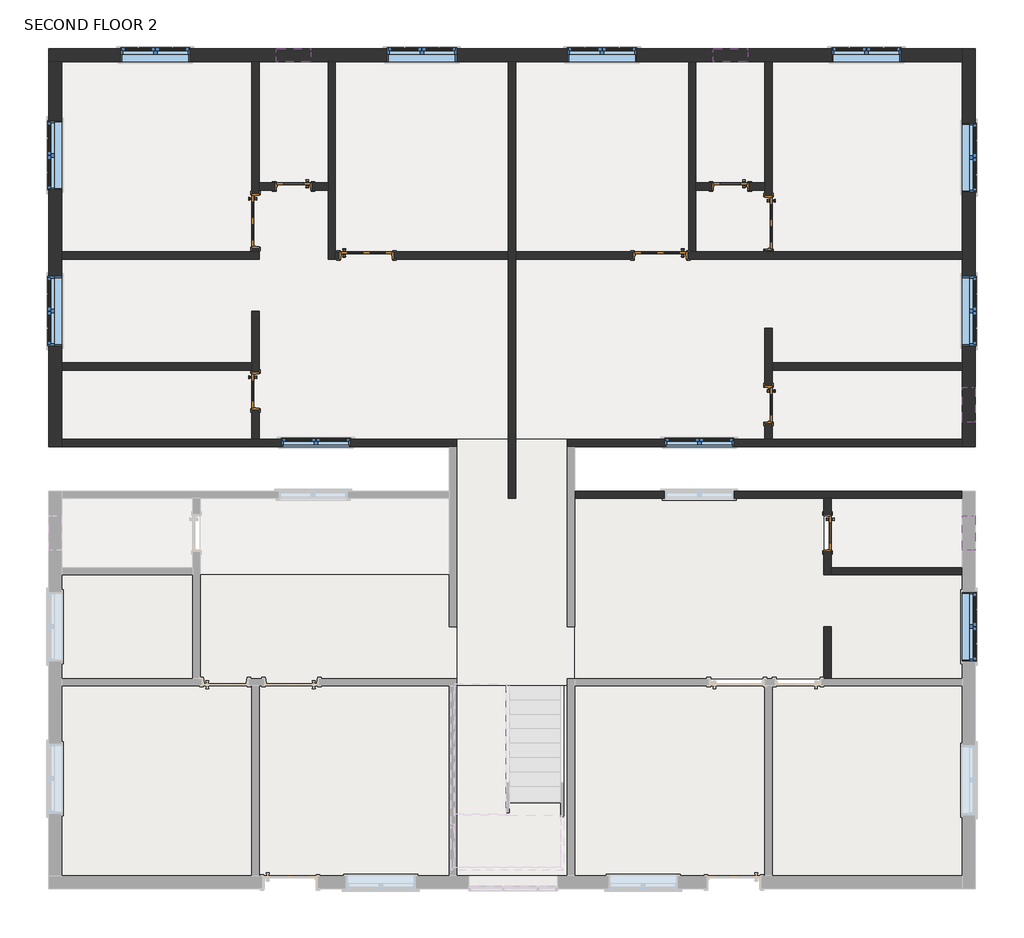
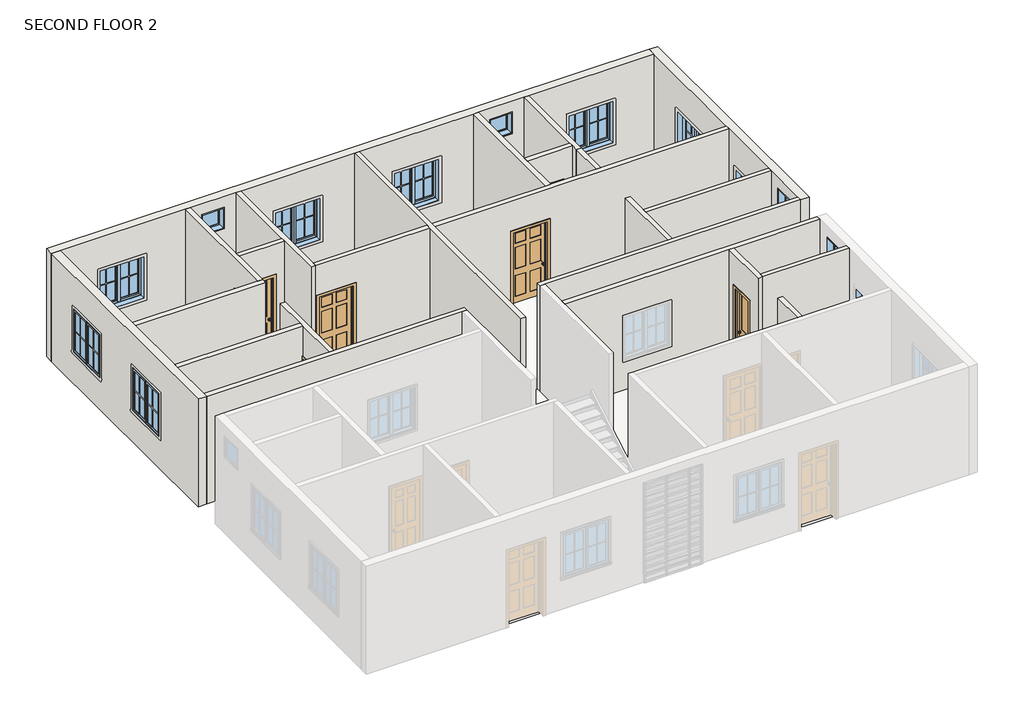
# One storey, part 3 of 4: 24 walls, 15 windows, 9 doors, 3 slabs.
"""IFC4 building model written with IfcOpenShell, lengths in millimetres."""

from ifc_helpers import new_model, si_unit, frame, origin, place, context, project, spatial, polyline, outline, extrude, faceted_brep, transform, mapped, element, save
from components import door_e337afa5, door_596d7c92, door_c610b25b, door_03e3dfb5, window_80340324, window_9200f5ac, window_c2c97eee

model = new_model("IFC4")

# Units and contexts
model_context = context("Model", 3, world=origin())
ifc_project = project(units=[si_unit("LENGTHUNIT", "METRE", prefix="MILLI")], contexts=[model_context])

# Site, building, storey
site = spatial("IfcSite", under=ifc_project)
building = spatial("IfcBuilding", under=site)
storey = spatial("IfcBuildingStorey", under=building, Name="SECOND FLOOR 2", Elevation=6343.9725604)

# Doors
placement = place(None, origin())
door_shape = door_e337afa5(model_context)
element("IfcDoor", 1, ObjectType="Door-Interior-Single-2_Panel-Wood : 24\" x 84\"", at=placement, inside=storey, context=model_context, shape_type="MappedRepresentation", body=[
    mapped(door_shape, transform((-8112.4137331, 4563.2156164, 6343.9725604), x_axis=(-1.0, 0.0, 0.0), y_axis=(0.0, -1.0, 0.0), z_axis=(0.0, 0.0, 1.0))),
])
element("IfcDoor", 2, ObjectType="Door-Interior-Single-2_Panel-Wood : 24\" x 84\"", at=placement, inside=storey, context=model_context, shape_type="MappedRepresentation", body=[
    mapped(door_shape, transform((-416.2137331, 4563.2156164, 6343.9725604), x_axis=(-1.0, 0.0, 0.0), y_axis=(0.0, -1.0, 0.0), z_axis=(0.0, 0.0, 1.0))),
])
element("IfcDoor", 3, ObjectType="Door-Interior-Single-2_Panel-Wood : 24\" x 84\"", at=placement, inside=storey, context=model_context, shape_type="MappedRepresentation", body=[
    mapped(door_shape, transform((-8788.6887331, 953.2406164, 6343.9725604), x_axis=(0.0, -1.0, 0.0), y_axis=(1.0, 0.0, 0.0), z_axis=(0.0, 0.0, 1.0))),
])
door_2_shape = door_596d7c92(model_context)
element("IfcDoor", 4, ObjectType="Door-Interior-Single-2_Panel-Wood : 24\" x 84\"", at=placement, inside=storey, context=model_context, shape_type="MappedRepresentation", body=[
    mapped(door_2_shape, transform((260.0612669, 711.9406164, 6343.9725604), x_axis=(0.0, -1.0, 0.0), y_axis=(1.0, 0.0, 0.0), z_axis=(0.0, 0.0, 1.0))),
])
element("IfcDoor", 5, ObjectType="Door-Interior-Single-2_Panel-Wood : 24\" x 84\"", at=placement, inside=storey, context=model_context, shape_type="MappedRepresentation", body=[
    mapped(door_2_shape, transform((1301.4612669, -1548.6593836, 6343.9725604), x_axis=(0.0, -1.0, 0.0), y_axis=(1.0, 0.0, 0.0), z_axis=(0.0, 0.0, 1.0))),
])
door_3_shape = door_c610b25b(model_context)
element("IfcDoor", 6, ObjectType="Door-Interior-Single-6_Panel-Wood : 36\" x 84\"", at=placement, inside=storey, context=model_context, shape_type="MappedRepresentation", body=[
    mapped(door_3_shape, transform((-8788.6887331, 3950.4406164, 6343.9725604), x_axis=(0.0, -1.0, 0.0), y_axis=(1.0, 0.0, 0.0), z_axis=(0.0, 0.0, 1.0))),
])
element("IfcDoor", 7, ObjectType="Door-Interior-Single-6_Panel-Wood : 36\" x 84\"", at=placement, inside=storey, context=model_context, shape_type="MappedRepresentation", body=[
    mapped(door_3_shape, transform((-1648.1137331, 3344.0156164, 6343.9725604), x_axis=(-1.0, 0.0, 0.0), y_axis=(0.0, -1.0, 0.0), z_axis=(0.0, 0.0, 1.0))),
])
door_4_shape = door_03e3dfb5(model_context)
element("IfcDoor", 8, ObjectType="Door-Interior-Single-6_Panel-Wood : 36\" x 84\"", at=placement, inside=storey, context=model_context, shape_type="MappedRepresentation", body=[
    mapped(door_4_shape, transform((-6829.7137331, 3344.0156164, 6343.9725604), x_axis=(1.0, 0.0, 0.0), y_axis=(0.0, 1.0, 0.0), z_axis=(0.0, 0.0, 1.0))),
])
element("IfcDoor", 9, ObjectType="Door-Interior-Single-6_Panel-Wood : 36\" x 84\"", at=placement, inside=storey, context=model_context, shape_type="MappedRepresentation", body=[
    mapped(door_4_shape, transform((260.0612669, 3912.3406164, 6343.9725604), x_axis=(0.0, -1.0, 0.0), y_axis=(1.0, 0.0, 0.0), z_axis=(0.0, 0.0, 1.0))),
])

# Slabs
element("IfcSlab", 10, ObjectType="marble tiles", at=placement, inside=storey, context=model_context, shape_type="SweptSolid", body=[
    extrude(outline(polyline([(-5242.2137331, -7593.8593836), (-12201.8137331, -7593.8593836), (-12201.8137331, -2285.2593836), (-5242.2137331, -2285.2593836), (-5242.2137331, -7593.8593836)])), frame((0.0, 0.0, 6248.4), z_axis=(0.0, 0.0, 1.0), x_axis=(1.0, 0.0, 0.0)), (0.0, 0.0, 1.0), 152.4),
])
element("IfcSlab", 11, ObjectType="marble tiles", at=placement, inside=storey, context=model_context, shape_type="SweptSolid", body=[
    extrude(outline(polyline([(-3159.4137331, -4241.0593836), (-5242.2137331, -4241.0593836), (-5242.2137331, 102.3406164), (-3159.4137331, 102.3406164), (-3159.4137331, -4241.0593836)])), frame((0.0, 0.0, 6248.4), z_axis=(0.0, 0.0, 1.0), x_axis=(1.0, 0.0, 0.0)), (0.0, 0.0, 1.0), 152.4),
])
element("IfcSlab", 12, ObjectType="marble tiles", at=placement, inside=storey, context=model_context, shape_type="SweptSolid", body=[
    extrude(outline(polyline([(-3286.4137331, -7593.8593836), (-5242.2137331, -7593.8593836), (-5242.2137331, -4241.0593836), (-3286.4137331, -4241.0593836), (-3286.4137331, -7593.8593836)])), frame((0.0, 0.0, 6248.4), z_axis=(0.0, 0.0, 1.0), x_axis=(1.0, 0.0, 0.0)), (0.0, 0.0, 1.0), 152.4),
    extrude(outline(polyline([(193.3862669, -7593.8593836), (-3159.4137331, -7593.8593836), (-3159.4137331, -4241.0593836), (193.3862669, -4241.0593836), (193.3862669, -7593.8593836)])), frame((0.0, 0.0, 6248.4), z_axis=(0.0, 0.0, 1.0), x_axis=(1.0, 0.0, 0.0)), (0.0, 0.0, 1.0), 152.4),
    extrude(outline(polyline([(3673.1862669, -7593.8593836), (320.3862669, -7593.8593836), (320.3862669, -4241.0593836), (3673.1862669, -4241.0593836), (3673.1862669, -7593.8593836)])), frame((0.0, 0.0, 6248.4), z_axis=(0.0, 0.0, 1.0), x_axis=(1.0, 0.0, 0.0)), (0.0, 0.0, 1.0), 152.4),
    extrude(outline(polyline([(1234.7862669, -4114.0593836), (-3159.4137331, -4114.0593836), (-3159.4137331, -939.0593836), (1234.7862669, -939.0593836), (1234.7862669, -2285.2593836), (3673.1862669, -2285.2593836), (3673.1862669, -4114.0593836), (1234.7862669, -4114.0593836)])), frame((0.0, 0.0, 6248.4), z_axis=(0.0, 0.0, 1.0), x_axis=(1.0, 0.0, 0.0)), (0.0, 0.0, 1.0), 152.4),
])

# Walls
element("IfcWall", 13, ObjectType="Inner Wall 5\"", at=placement, inside=storey, context=model_context, shape_type="Brep", body=[
    faceted_brep([(-12201.8137331, -24.6593836, 6343.9725604), (-5369.2137331, -24.6593836, 6343.9725604), (-5242.2137331, -24.6593836, 6343.9725604), (-5242.2137331, -24.6593836, 9391.9725604), (-5369.2137331, -24.6593836, 9391.9725604), (-12201.8137331, -24.6593836, 9391.9725604), (-7109.1137331, -24.6593836, 8477.5725604), (-7109.1137331, -24.6593836, 7258.3725604), (-8328.3137331, -24.6593836, 7258.3725604), (-8328.3137331, -24.6593836, 8477.5725604), (-12201.8137331, 102.3406164, 6343.9725604), (-12201.8137331, 102.3406164, 9391.9725604), (-8849.0137331, 102.3406164, 9391.9725604), (-8722.0137331, 102.3406164, 9391.9725604), (-5242.2137331, 102.3406164, 9391.9725604), (-5242.2137331, 102.3406164, 6343.9725604), (-8722.0137331, 102.3406164, 6343.9725604), (-8849.0137331, 102.3406164, 6343.9725604), (-7109.1137331, 102.3406164, 8477.5725604), (-8328.3137331, 102.3406164, 8477.5725604), (-8328.3137331, 102.3406164, 7258.3725604), (-7109.1137331, 102.3406164, 7258.3725604)], [[[0, 1, 2, 3, 4, 5], [6, 7, 8, 9]], [[10, 11, 12, 13, 14, 15, 16, 17], [18, 19, 20, 21]], [[2, 1, 0, 10, 17, 16, 15]], [[5, 4, 3, 14, 13, 12, 11]], [[0, 5, 11, 10]], [[3, 2, 15, 14]], [[7, 6, 18, 21]], [[8, 7, 21, 20]], [[9, 8, 20, 19]], [[6, 9, 19, 18]]]),
])
element("IfcWall", 14, ObjectType="Inner Wall 5\"", at=placement, inside=storey, context=model_context, shape_type="Brep", body=[
    faceted_brep([(3673.1862669, 102.3406164, 6343.9725604), (320.3862669, 102.3406164, 6343.9725604), (193.3862669, 102.3406164, 6343.9725604), (-3286.4137331, 102.3406164, 6343.9725604), (-3286.4137331, 102.3406164, 9391.9725604), (193.3862669, 102.3406164, 9391.9725604), (320.3862669, 102.3406164, 9391.9725604), (3673.1862669, 102.3406164, 9391.9725604), (-352.7137331, 102.3406164, 8477.5725604), (-1571.9137331, 102.3406164, 8477.5725604), (-1571.9137331, 102.3406164, 7258.3725604), (-352.7137331, 102.3406164, 7258.3725604), (3673.1862669, -24.6593836, 6343.9725604), (3673.1862669, -24.6593836, 9391.9725604), (-3159.4137331, -24.6593836, 9391.9725604), (-3286.4137331, -24.6593836, 9391.9725604), (-3286.4137331, -24.6593836, 6343.9725604), (-3159.4137331, -24.6593836, 6343.9725604), (-352.7137331, -24.6593836, 8477.5725604), (-352.7137331, -24.6593836, 7258.3725604), (-1571.9137331, -24.6593836, 7258.3725604), (-1571.9137331, -24.6593836, 8477.5725604)], [[[0, 1, 2, 3, 4, 5, 6, 7], [8, 9, 10, 11]], [[12, 13, 14, 15, 16, 17], [18, 19, 20, 21]], [[3, 2, 1, 0, 12, 17, 16]], [[7, 6, 5, 4, 15, 14, 13]], [[0, 7, 13, 12]], [[4, 3, 16, 15]], [[19, 18, 8, 11]], [[20, 19, 11, 10]], [[21, 20, 10, 9]], [[18, 21, 9, 8]]]),
])
element("IfcWall", 15, ObjectType="Inner Wall 5\"", at=placement, inside=storey, context=model_context, shape_type="Brep", body=[
    faceted_brep([(3673.1862669, -812.0593836, 6343.9725604), (-3159.4137331, -812.0593836, 6343.9725604), (-3159.4137331, -812.0593836, 9391.9725604), (3673.1862669, -812.0593836, 9391.9725604), (-352.7137331, -812.0593836, 8477.5725604), (-1571.9137331, -812.0593836, 8477.5725604), (-1571.9137331, -812.0593836, 7258.3725604), (-352.7137331, -812.0593836, 7258.3725604), (3673.1862669, -939.0593836, 6343.9725604), (3673.1862669, -939.0593836, 9391.9725604), (1361.7862669, -939.0593836, 9391.9725604), (1234.7862669, -939.0593836, 9391.9725604), (-3159.4137331, -939.0593836, 9391.9725604), (-3159.4137331, -939.0593836, 6343.9725604), (1234.7862669, -939.0593836, 6343.9725604), (1361.7862669, -939.0593836, 6343.9725604), (-352.7137331, -939.0593836, 8477.5725604), (-352.7137331, -939.0593836, 7258.3725604), (-1571.9137331, -939.0593836, 7258.3725604), (-1571.9137331, -939.0593836, 8477.5725604)], [[[0, 1, 2, 3], [4, 5, 6, 7]], [[8, 9, 10, 11, 12, 13, 14, 15], [16, 17, 18, 19]], [[1, 0, 8, 15, 14, 13]], [[3, 2, 12, 11, 10, 9]], [[0, 3, 9, 8]], [[2, 1, 13, 12]], [[17, 16, 4, 7]], [[18, 17, 7, 6]], [[19, 18, 6, 5]], [[16, 19, 5, 4]]]),
])
element("IfcWall", 16, ObjectType="Inner Wall 5\"", at=placement, inside=storey, context=model_context, shape_type="Brep", body=[
    faceted_brep([(1234.7862669, -2285.2593836, 9391.9725604), (1234.7862669, -939.0593836, 9391.9725604), (1234.7862669, -939.0593836, 6343.9725604), (1234.7862669, -1218.4593836, 6343.9725604), (1234.7862669, -1218.4593836, 8502.9725604), (1234.7862669, -1878.8593836, 8502.9725604), (1234.7862669, -1878.8593836, 6343.9725604), (1234.7862669, -2285.2593836, 6343.9725604), (1361.7862669, -939.0593836, 9391.9725604), (1361.7862669, -2158.2593836, 9391.9725604), (1361.7862669, -2285.2593836, 9391.9725604), (1361.7862669, -2285.2593836, 6343.9725604), (1361.7862669, -2158.2593836, 6343.9725604), (1361.7862669, -1878.8593836, 6343.9725604), (1361.7862669, -1878.8593836, 8502.9725604), (1361.7862669, -1218.4593836, 8502.9725604), (1361.7862669, -1218.4593836, 6343.9725604), (1361.7862669, -939.0593836, 6343.9725604)], [[[0, 1, 2, 3, 4, 5, 6, 7]], [[8, 9, 10, 11, 12, 13, 14, 15, 16, 17]], [[2, 17, 16, 3]], [[11, 7, 6, 13, 12]], [[1, 0, 10, 9, 8]], [[2, 1, 8, 17]], [[0, 7, 11, 10]], [[5, 14, 13, 6]], [[14, 5, 4, 15]], [[15, 4, 3, 16]]]),
])
element("IfcWall", 17, ObjectType="Inner Wall 5\"", at=placement, inside=storey, context=model_context, shape_type="SweptSolid", body=[
    extrude(outline(polyline([(3673.1862669, -2285.2593836), (1361.7862669, -2285.2593836), (1361.7862669, -2158.2593836), (3673.1862669, -2158.2593836), (3673.1862669, -2285.2593836)])), frame((0.0, 0.0, 6343.9725604), z_axis=(0.0, 0.0, 1.0), x_axis=(1.0, 0.0, 0.0)), (0.0, 0.0, 1.0), 3048.0),
])
element("IfcWall", 18, ObjectType="Inner Wall 5\"", at=placement, inside=storey, context=model_context, shape_type="SweptSolid", body=[
    extrude(outline(polyline([(1361.7862669, -3199.6593836), (1361.7862669, -4114.0593836), (1234.7862669, -4114.0593836), (1234.7862669, -3199.6593836), (1361.7862669, -3199.6593836)])), frame((0.0, 0.0, 6343.9725604), z_axis=(0.0, 0.0, 1.0), x_axis=(1.0, 0.0, 0.0)), (0.0, 0.0, 1.0), 3048.0),
])
element("IfcWall", 19, ObjectType="Inner Wall 5\"", at=placement, inside=storey, context=model_context, shape_type="Brep", body=[
    faceted_brep([(-12201.8137331, 3277.3406164, 6343.9725604), (-8722.0137331, 3277.3406164, 6343.9725604), (-8722.0137331, 3277.3406164, 9391.9725604), (-12201.8137331, 3277.3406164, 9391.9725604), (-12201.8137331, 3404.3406164, 6343.9725604), (-12201.8137331, 3404.3406164, 9391.9725604), (-8849.0137331, 3404.3406164, 9391.9725604), (-8722.0137331, 3404.3406164, 9391.9725604), (-8722.0137331, 3404.3406164, 6343.9725604), (-8849.0137331, 3404.3406164, 6343.9725604)], [[[0, 1, 2, 3]], [[4, 5, 6, 7, 8, 9]], [[1, 0, 4, 9, 8]], [[3, 2, 7, 6, 5]], [[0, 3, 5, 4]], [[2, 1, 8, 7]]]),
])
element("IfcWall", 20, ObjectType="Inner Wall 5\"", at=placement, inside=storey, context=model_context, shape_type="Brep", body=[
    faceted_brep([(-8722.0137331, 6758.7281164, 9391.9725604), (-8722.0137331, 4623.5406164, 9391.9725604), (-8722.0137331, 4496.5406164, 9391.9725604), (-8722.0137331, 3404.3406164, 9391.9725604), (-8722.0137331, 3404.3406164, 6343.9725604), (-8722.0137331, 3467.8406164, 6343.9725604), (-8722.0137331, 3467.8406164, 8502.9725604), (-8722.0137331, 4433.0406164, 8502.9725604), (-8722.0137331, 4433.0406164, 6343.9725604), (-8722.0137331, 4496.5406164, 6343.9725604), (-8722.0137331, 4623.5406164, 6343.9725604), (-8722.0137331, 6758.7281164, 6343.9725604), (-8849.0137331, 3404.3406164, 9391.9725604), (-8849.0137331, 6758.7281164, 9391.9725604), (-8849.0137331, 6758.7281164, 6343.9725604), (-8849.0137331, 4433.0406164, 6343.9725604), (-8849.0137331, 4433.0406164, 8502.9725604), (-8849.0137331, 3467.8406164, 8502.9725604), (-8849.0137331, 3467.8406164, 6343.9725604), (-8849.0137331, 3404.3406164, 6343.9725604)], [[[0, 1, 2, 3, 4, 5, 6, 7, 8, 9, 10, 11]], [[12, 13, 14, 15, 16, 17, 18, 19]], [[4, 19, 18, 5]], [[14, 11, 10, 9, 8, 15]], [[3, 2, 1, 0, 13, 12]], [[4, 3, 12, 19]], [[0, 11, 14, 13]], [[17, 6, 5, 18]], [[6, 17, 16, 7]], [[7, 16, 15, 8]]]),
])
element("IfcWall", 21, ObjectType="Inner Wall 5\"", at=placement, inside=storey, context=model_context, shape_type="SweptSolid", body=[
    extrude(outline(polyline([(9391.9725604, -7502.8137331), (9391.9725604, -8722.0137331), (6343.9725604, -8722.0137331), (6343.9725604, -8442.6137331), (8502.9725604, -8442.6137331), (8502.9725604, -7782.2137331), (6343.9725604, -7782.2137331), (6343.9725604, -7502.8137331), (9391.9725604, -7502.8137331)])), frame((0.0, 4496.5406164, 0.0), z_axis=(0.0, 1.0, 0.0), x_axis=(0.0, 0.0, 1.0)), (0.0, 0.0, 1.0), 127.0),
])
element("IfcWall", 22, ObjectType="Inner Wall 5\"", at=placement, inside=storey, context=model_context, shape_type="Brep", body=[
    faceted_brep([(-7375.8137331, 3277.3406164, 6343.9725604), (-7375.8137331, 3404.3406164, 6343.9725604), (-7375.8137331, 6758.7281164, 6343.9725604), (-7375.8137331, 6758.7281164, 9391.9725604), (-7375.8137331, 3404.3406164, 9391.9725604), (-7375.8137331, 3277.3406164, 9391.9725604), (-7502.8137331, 3277.3406164, 6343.9725604), (-7502.8137331, 3277.3406164, 9391.9725604), (-7502.8137331, 4496.5406164, 9391.9725604), (-7502.8137331, 4623.5406164, 9391.9725604), (-7502.8137331, 6758.7281164, 9391.9725604), (-7502.8137331, 6758.7281164, 6343.9725604), (-7502.8137331, 4623.5406164, 6343.9725604), (-7502.8137331, 4496.5406164, 6343.9725604)], [[[0, 1, 2, 3, 4, 5]], [[6, 7, 8, 9, 10, 11, 12, 13]], [[2, 1, 0, 6, 13, 12, 11]], [[5, 4, 3, 10, 9, 8, 7]], [[3, 2, 11, 10]], [[0, 5, 7, 6]]]),
])
element("IfcWall", 23, ObjectType="Inner Wall 5\"", at=placement, inside=storey, context=model_context, shape_type="Brep", body=[
    faceted_brep([(-4327.8137331, 6758.7281164, 6343.9725604), (-4327.8137331, 3404.3406164, 6343.9725604), (-4327.8137331, 3277.3406164, 6343.9725604), (-4327.8137331, -939.0593836, 6343.9725604), (-4327.8137331, -939.0593836, 9391.9725604), (-4327.8137331, 3277.3406164, 9391.9725604), (-4327.8137331, 3404.3406164, 9391.9725604), (-4327.8137331, 6758.7281164, 9391.9725604), (-4200.8137331, 6758.7281164, 6343.9725604), (-4200.8137331, 6758.7281164, 9391.9725604), (-4200.8137331, 3404.3406164, 9391.9725604), (-4200.8137331, 3277.3406164, 9391.9725604), (-4200.8137331, -939.0593836, 9391.9725604), (-4200.8137331, -939.0593836, 6343.9725604), (-4200.8137331, 3277.3406164, 6343.9725604), (-4200.8137331, 3404.3406164, 6343.9725604)], [[[0, 1, 2, 3, 4, 5, 6, 7]], [[8, 9, 10, 11, 12, 13, 14, 15]], [[3, 2, 1, 0, 8, 15, 14, 13]], [[4, 3, 13, 12]], [[7, 6, 5, 4, 12, 11, 10, 9]], [[0, 7, 9, 8]]]),
])
element("IfcWall", 24, ObjectType="Inner Wall 5\"", at=placement, inside=storey, context=model_context, shape_type="SweptSolid", body=[
    extrude(outline(polyline([(9391.9725604, -4327.8137331), (9391.9725604, -7375.8137331), (6343.9725604, -7375.8137331), (6343.9725604, -7312.3137331), (8502.9725604, -7312.3137331), (8502.9725604, -6347.1137331), (6343.9725604, -6347.1137331), (6343.9725604, -4327.8137331), (9391.9725604, -4327.8137331)])), frame((0.0, 3277.3406164, 0.0), z_axis=(0.0, 1.0, 0.0), x_axis=(0.0, 0.0, 1.0)), (0.0, 0.0, 1.0), 127.0),
])
element("IfcWall", 25, ObjectType="Inner Wall 5\"", at=placement, inside=storey, context=model_context, shape_type="Brep", body=[
    faceted_brep([(3673.1862669, 3277.3406164, 9391.9725604), (-4200.8137331, 3277.3406164, 9391.9725604), (-4200.8137331, 3277.3406164, 6343.9725604), (-2130.7137331, 3277.3406164, 6343.9725604), (-2130.7137331, 3277.3406164, 8502.9725604), (-1165.5137331, 3277.3406164, 8502.9725604), (-1165.5137331, 3277.3406164, 6343.9725604), (3673.1862669, 3277.3406164, 6343.9725604), (-4200.8137331, 3404.3406164, 9391.9725604), (-1152.8137331, 3404.3406164, 9391.9725604), (-1025.8137331, 3404.3406164, 9391.9725604), (193.3862669, 3404.3406164, 9391.9725604), (320.3862669, 3404.3406164, 9391.9725604), (3673.1862669, 3404.3406164, 9391.9725604), (3673.1862669, 3404.3406164, 6343.9725604), (320.3862669, 3404.3406164, 6343.9725604), (193.3862669, 3404.3406164, 6343.9725604), (-1025.8137331, 3404.3406164, 6343.9725604), (-1152.8137331, 3404.3406164, 6343.9725604), (-1165.5137331, 3404.3406164, 6343.9725604), (-1165.5137331, 3404.3406164, 8502.9725604), (-2130.7137331, 3404.3406164, 8502.9725604), (-2130.7137331, 3404.3406164, 6343.9725604), (-4200.8137331, 3404.3406164, 6343.9725604)], [[[0, 1, 2, 3, 4, 5, 6, 7]], [[8, 9, 10, 11, 12, 13, 14, 15, 16, 17, 18, 19, 20, 21, 22, 23]], [[2, 23, 22, 3]], [[14, 7, 6, 19, 18, 17, 16, 15]], [[1, 0, 13, 12, 11, 10, 9, 8]], [[2, 1, 8, 23]], [[0, 7, 14, 13]], [[21, 4, 3, 22]], [[4, 21, 20, 5]], [[5, 20, 19, 6]]]),
])
element("IfcWall", 26, ObjectType="Inner Wall 5\"", at=placement, inside=storey, context=model_context, shape_type="Brep", body=[
    faceted_brep([(-1025.8137331, 3404.3406164, 6343.9725604), (-1025.8137331, 4496.5406164, 6343.9725604), (-1025.8137331, 4623.5406164, 6343.9725604), (-1025.8137331, 6758.7281164, 6343.9725604), (-1025.8137331, 6758.7281164, 9391.9725604), (-1025.8137331, 4623.5406164, 9391.9725604), (-1025.8137331, 4496.5406164, 9391.9725604), (-1025.8137331, 3404.3406164, 9391.9725604), (-1152.8137331, 3404.3406164, 6343.9725604), (-1152.8137331, 3404.3406164, 9391.9725604), (-1152.8137331, 6758.7281164, 9391.9725604), (-1152.8137331, 6758.7281164, 6343.9725604)], [[[0, 1, 2, 3, 4, 5, 6, 7]], [[8, 9, 10, 11]], [[3, 2, 1, 0, 8, 11]], [[7, 6, 5, 4, 10, 9]], [[0, 7, 9, 8]], [[4, 3, 11, 10]]]),
])
element("IfcWall", 27, ObjectType="Inner Wall 5\"", at=placement, inside=storey, context=model_context, shape_type="SweptSolid", body=[
    extrude(outline(polyline([(9391.9725604, 193.3862669), (9391.9725604, -1025.8137331), (6343.9725604, -1025.8137331), (6343.9725604, -746.4137331), (8502.9725604, -746.4137331), (8502.9725604, -86.0137331), (6343.9725604, -86.0137331), (6343.9725604, 193.3862669), (9391.9725604, 193.3862669)])), frame((0.0, 4496.5406164, 0.0), z_axis=(0.0, 1.0, 0.0), x_axis=(0.0, 0.0, 1.0)), (0.0, 0.0, 1.0), 127.0),
])
element("IfcWall", 28, ObjectType="Inner Wall 5\"", at=placement, inside=storey, context=model_context, shape_type="Brep", body=[
    faceted_brep([(320.3862669, 6758.7281164, 9391.9725604), (320.3862669, 4318.7406164, 9391.9725604), (320.3862669, 4318.7406164, 8502.9725604), (320.3862669, 4394.9406164, 8502.9725604), (320.3862669, 4394.9406164, 6343.9725604), (320.3862669, 6758.7281164, 6343.9725604), (193.3862669, 4318.7406164, 9391.9725604), (193.3862669, 4496.5406164, 9391.9725604), (193.3862669, 4623.5406164, 9391.9725604), (193.3862669, 6758.7281164, 9391.9725604), (193.3862669, 6758.7281164, 6343.9725604), (193.3862669, 4623.5406164, 6343.9725604), (193.3862669, 4496.5406164, 6343.9725604), (193.3862669, 4394.9406164, 6343.9725604), (193.3862669, 4394.9406164, 8502.9725604), (193.3862669, 4318.7406164, 8502.9725604)], [[[0, 1, 2, 3, 4, 5]], [[6, 7, 8, 9, 10, 11, 12, 13, 14, 15]], [[10, 5, 4, 13, 12, 11]], [[1, 0, 9, 8, 7, 6]], [[1, 6, 15, 2]], [[0, 5, 10, 9]], [[14, 3, 2, 15]], [[3, 14, 13, 4]]]),
])
element("IfcWall", 29, ObjectType="Inner Wall 5\"", at=placement, inside=storey, context=model_context, shape_type="SweptSolid", body=[
    extrude(outline(polyline([(320.3862669, 1448.5406164), (3673.1862669, 1448.5406164), (3673.1862669, 1321.5406164), (320.3862669, 1321.5406164), (320.3862669, 1448.5406164)])), frame((0.0, 0.0, 6343.9725604), z_axis=(0.0, 0.0, 1.0), x_axis=(1.0, 0.0, 0.0)), (0.0, 0.0, 1.0), 3048.0),
])
element("IfcWall", 30, ObjectType="Inner Wall 5\"", at=placement, inside=storey, context=model_context, shape_type="Brep", body=[
    faceted_brep([(193.3862669, 102.3406164, 9391.9725604), (193.3862669, 2058.1406164, 9391.9725604), (193.3862669, 2058.1406164, 6343.9725604), (193.3862669, 1042.1406164, 6343.9725604), (193.3862669, 1042.1406164, 8502.9725604), (193.3862669, 381.7406164, 8502.9725604), (193.3862669, 381.7406164, 6343.9725604), (193.3862669, 102.3406164, 6343.9725604), (320.3862669, 2058.1406164, 9391.9725604), (320.3862669, 1448.5406164, 9391.9725604), (320.3862669, 1321.5406164, 9391.9725604), (320.3862669, 102.3406164, 9391.9725604), (320.3862669, 102.3406164, 6343.9725604), (320.3862669, 381.7406164, 6343.9725604), (320.3862669, 381.7406164, 8502.9725604), (320.3862669, 1042.1406164, 8502.9725604), (320.3862669, 1042.1406164, 6343.9725604), (320.3862669, 1321.5406164, 6343.9725604), (320.3862669, 1448.5406164, 6343.9725604), (320.3862669, 2058.1406164, 6343.9725604)], [[[0, 1, 2, 3, 4, 5, 6, 7]], [[8, 9, 10, 11, 12, 13, 14, 15, 16, 17, 18, 19]], [[2, 19, 18, 17, 16, 3]], [[12, 7, 6, 13]], [[1, 0, 11, 10, 9, 8]], [[2, 1, 8, 19]], [[0, 7, 12, 11]], [[5, 14, 13, 6]], [[14, 5, 4, 15]], [[15, 4, 3, 16]]]),
])
element("IfcWall", 31, ObjectType="Inner Wall 5\"", at=placement, inside=storey, context=model_context, shape_type="Brep", body=[
    faceted_brep([(-8722.0137331, 2362.9406164, 6343.9725604), (-8722.0137331, 2362.9406164, 9391.9725604), (-8722.0137331, 102.3406164, 9391.9725604), (-8722.0137331, 102.3406164, 6343.9725604), (-8722.0137331, 623.0406164, 6343.9725604), (-8722.0137331, 623.0406164, 8502.9725604), (-8722.0137331, 1283.4406164, 8502.9725604), (-8722.0137331, 1283.4406164, 6343.9725604), (-8849.0137331, 2362.9406164, 9391.9725604), (-8849.0137331, 2362.9406164, 6343.9725604), (-8849.0137331, 1448.5406164, 6343.9725604), (-8849.0137331, 1321.5406164, 6343.9725604), (-8849.0137331, 1283.4406164, 6343.9725604), (-8849.0137331, 1283.4406164, 8502.9725604), (-8849.0137331, 623.0406164, 8502.9725604), (-8849.0137331, 623.0406164, 6343.9725604), (-8849.0137331, 102.3406164, 6343.9725604), (-8849.0137331, 102.3406164, 9391.9725604), (-8849.0137331, 1321.5406164, 9391.9725604), (-8849.0137331, 1448.5406164, 9391.9725604)], [[[0, 1, 2, 3, 4, 5, 6, 7]], [[8, 9, 10, 11, 12, 13, 14, 15, 16, 17, 18, 19]], [[9, 0, 7, 12, 11, 10]], [[3, 16, 15, 4]], [[1, 0, 9, 8]], [[2, 1, 8, 19, 18, 17]], [[3, 2, 17, 16]], [[14, 5, 4, 15]], [[5, 14, 13, 6]], [[6, 13, 12, 7]]]),
])
element("IfcWall", 32, ObjectType="Inner Wall 5\"", at=placement, inside=storey, context=model_context, shape_type="SweptSolid", body=[
    extrude(outline(polyline([(-12201.8137331, 1448.5406164), (-8849.0137331, 1448.5406164), (-8849.0137331, 1321.5406164), (-12201.8137331, 1321.5406164), (-12201.8137331, 1448.5406164)])), frame((0.0, 0.0, 6343.9725604), z_axis=(0.0, 0.0, 1.0), x_axis=(1.0, 0.0, 0.0)), (0.0, 0.0, 1.0), 3048.0),
])
element("IfcWall", 33, ObjectType="Inner Wall 5\"", at=placement, inside=storey, context=model_context, shape_type="SweptSolid", body=[
    extrude(outline(polyline([(3404.3406164, 9391.9725604), (4318.7406164, 9391.9725604), (4318.7406164, 8502.9725604), (3429.7406164, 8502.9725604), (3429.7406164, 6343.9725604), (3404.3406164, 6343.9725604), (3404.3406164, 9391.9725604)])), frame((193.3862669, 0.0, 0.0), z_axis=(1.0, 0.0, 0.0), x_axis=(0.0, 1.0, 0.0)), (0.0, 0.0, 1.0), 127.0),
])
element("IfcWall", 34, ObjectType="outer wall 9\"", at=placement, inside=storey, context=model_context, shape_type="Brep", body=[
    faceted_brep([(-12430.4137331, 6758.7281164, 6343.9725604), (-12201.8137331, 6758.7281164, 6343.9725604), (-8849.0137331, 6758.7281164, 6343.9725604), (-8722.0137331, 6758.7281164, 6343.9725604), (-7502.8137331, 6758.7281164, 6343.9725604), (-7375.8137331, 6758.7281164, 6343.9725604), (-4327.8137331, 6758.7281164, 6343.9725604), (-4200.8137331, 6758.7281164, 6343.9725604), (-1152.8137331, 6758.7281164, 6343.9725604), (-1025.8137331, 6758.7281164, 6343.9725604), (193.3862669, 6758.7281164, 6343.9725604), (320.3862669, 6758.7281164, 6343.9725604), (3673.1862669, 6758.7281164, 6343.9725604), (3673.1862669, 6758.7281164, 9391.9725604), (320.3862669, 6758.7281164, 9391.9725604), (193.3862669, 6758.7281164, 9391.9725604), (-1025.8137331, 6758.7281164, 9391.9725604), (-1152.8137331, 6758.7281164, 9391.9725604), (-4200.8137331, 6758.7281164, 9391.9725604), (-4327.8137331, 6758.7281164, 9391.9725604), (-7375.8137331, 6758.7281164, 9391.9725604), (-7502.8137331, 6758.7281164, 9391.9725604), (-8722.0137331, 6758.7281164, 9391.9725604), (-8849.0137331, 6758.7281164, 9391.9725604), (-12201.8137331, 6758.7281164, 9391.9725604), (-12430.4137331, 6758.7281164, 9391.9725604), (-9941.2137331, 6758.7281164, 8477.5725604), (-9941.2137331, 6758.7281164, 7258.3725604), (-11160.4137331, 6758.7281164, 7258.3725604), (-11160.4137331, 6758.7281164, 8477.5725604), (-5242.2137331, 6758.7281164, 8477.5725604), (-5242.2137331, 6758.7281164, 7258.3725604), (-6461.4137331, 6758.7281164, 7258.3725604), (-6461.4137331, 6758.7281164, 8477.5725604), (-2067.2137331, 6758.7281164, 8477.5725604), (-2067.2137331, 6758.7281164, 7258.3725604), (-3286.4137331, 6758.7281164, 7258.3725604), (-3286.4137331, 6758.7281164, 8477.5725604), (2593.6862669, 6758.7281164, 8477.5725604), (2593.6862669, 6758.7281164, 7258.3725604), (1374.4862669, 6758.7281164, 7258.3725604), (1374.4862669, 6758.7281164, 8477.5725604), (-7807.6137331, 6758.7281164, 9087.1725604), (-7807.6137331, 6758.7281164, 8477.5725604), (-8417.2137331, 6758.7281164, 8477.5725604), (-8417.2137331, 6758.7281164, 9087.1725604), (-111.4137331, 6758.7281164, 9087.1725604), (-111.4137331, 6758.7281164, 8477.5725604), (-721.0137331, 6758.7281164, 8477.5725604), (-721.0137331, 6758.7281164, 9087.1725604), (-12430.4137331, 6987.3281164, 6343.9725604), (-12430.4137331, 6987.3281164, 9391.9725604), (3673.1862669, 6987.3281164, 9391.9725604), (3673.1862669, 6987.3281164, 6343.9725604), (-9941.2137331, 6987.3281164, 8477.5725604), (-11160.4137331, 6987.3281164, 8477.5725604), (-11160.4137331, 6987.3281164, 7258.3725604), (-9941.2137331, 6987.3281164, 7258.3725604), (-5242.2137331, 6987.3281164, 8477.5725604), (-6461.4137331, 6987.3281164, 8477.5725604), (-6461.4137331, 6987.3281164, 7258.3725604), (-5242.2137331, 6987.3281164, 7258.3725604), (-2067.2137331, 6987.3281164, 8477.5725604), (-3286.4137331, 6987.3281164, 8477.5725604), (-3286.4137331, 6987.3281164, 7258.3725604), (-2067.2137331, 6987.3281164, 7258.3725604), (2593.6862669, 6987.3281164, 8477.5725604), (1374.4862669, 6987.3281164, 8477.5725604), (1374.4862669, 6987.3281164, 7258.3725604), (2593.6862669, 6987.3281164, 7258.3725604), (-7807.6137331, 6987.3281164, 9087.1725604), (-8417.2137331, 6987.3281164, 9087.1725604), (-8417.2137331, 6987.3281164, 8477.5725604), (-7807.6137331, 6987.3281164, 8477.5725604), (-111.4137331, 6987.3281164, 9087.1725604), (-721.0137331, 6987.3281164, 9087.1725604), (-721.0137331, 6987.3281164, 8477.5725604), (-111.4137331, 6987.3281164, 8477.5725604)], [[[0, 1, 2, 3, 4, 5, 6, 7, 8, 9, 10, 11, 12, 13, 14, 15, 16, 17, 18, 19, 20, 21, 22, 23, 24, 25], [26, 27, 28, 29], [30, 31, 32, 33], [34, 35, 36, 37], [38, 39, 40, 41], [42, 43, 44, 45], [46, 47, 48, 49]], [[50, 51, 52, 53], [54, 55, 56, 57], [58, 59, 60, 61], [62, 63, 64, 65], [66, 67, 68, 69], [70, 71, 72, 73], [74, 75, 76, 77]], [[12, 11, 10, 9, 8, 7, 6, 5, 4, 3, 2, 1, 0, 50, 53]], [[25, 24, 23, 22, 21, 20, 19, 18, 17, 16, 15, 14, 13, 52, 51]], [[0, 25, 51, 50]], [[13, 12, 53, 52]], [[27, 26, 54, 57]], [[28, 27, 57, 56]], [[29, 28, 56, 55]], [[26, 29, 55, 54]], [[31, 30, 58, 61]], [[32, 31, 61, 60]], [[33, 32, 60, 59]], [[30, 33, 59, 58]], [[35, 34, 62, 65]], [[36, 35, 65, 64]], [[37, 36, 64, 63]], [[34, 37, 63, 62]], [[39, 38, 66, 69]], [[40, 39, 69, 68]], [[41, 40, 68, 67]], [[38, 41, 67, 66]], [[43, 42, 70, 73]], [[44, 43, 73, 72]], [[45, 44, 72, 71]], [[42, 45, 71, 70]], [[47, 46, 74, 77]], [[48, 47, 77, 76]], [[49, 48, 76, 75]], [[46, 49, 75, 74]]]),
])
element("IfcWall", 35, ObjectType="outer wall 9\"", at=placement, inside=storey, context=model_context, shape_type="Brep", body=[
    faceted_brep([(-12201.8137331, -24.6593836, 6343.9725604), (-12201.8137331, 102.3406164, 6343.9725604), (-12201.8137331, 1321.5406164, 6343.9725604), (-12201.8137331, 1448.5406164, 6343.9725604), (-12201.8137331, 3277.3406164, 6343.9725604), (-12201.8137331, 3404.3406164, 6343.9725604), (-12201.8137331, 6758.7281164, 6343.9725604), (-12201.8137331, 6758.7281164, 9391.9725604), (-12201.8137331, 3404.3406164, 9391.9725604), (-12201.8137331, 3277.3406164, 9391.9725604), (-12201.8137331, 1448.5406164, 9391.9725604), (-12201.8137331, 1321.5406164, 9391.9725604), (-12201.8137331, 102.3406164, 9391.9725604), (-12201.8137331, -24.6593836, 9391.9725604), (-12201.8137331, 2972.5406164, 8477.5725604), (-12201.8137331, 2972.5406164, 7258.3725604), (-12201.8137331, 1753.3406164, 7258.3725604), (-12201.8137331, 1753.3406164, 8477.5725604), (-12201.8137331, 5716.5343664, 8477.5725604), (-12201.8137331, 5716.5343664, 7258.3725604), (-12201.8137331, 4497.3343664, 7258.3725604), (-12201.8137331, 4497.3343664, 8477.5725604), (-12430.4137331, -24.6593836, 6343.9725604), (-12430.4137331, -24.6593836, 9391.9725604), (-12430.4137331, 6758.7281164, 9391.9725604), (-12430.4137331, 6758.7281164, 6343.9725604), (-12430.4137331, 2972.5406164, 8477.5725604), (-12430.4137331, 1753.3406164, 8477.5725604), (-12430.4137331, 1753.3406164, 7258.3725604), (-12430.4137331, 2972.5406164, 7258.3725604), (-12430.4137331, 5716.5343664, 8477.5725604), (-12430.4137331, 4497.3343664, 8477.5725604), (-12430.4137331, 4497.3343664, 7258.3725604), (-12430.4137331, 5716.5343664, 7258.3725604)], [[[0, 1, 2, 3, 4, 5, 6, 7, 8, 9, 10, 11, 12, 13], [14, 15, 16, 17], [18, 19, 20, 21]], [[22, 23, 24, 25], [26, 27, 28, 29], [30, 31, 32, 33]], [[6, 5, 4, 3, 2, 1, 0, 22, 25]], [[13, 12, 11, 10, 9, 8, 7, 24, 23]], [[7, 6, 25, 24]], [[0, 13, 23, 22]], [[15, 14, 26, 29]], [[16, 15, 29, 28]], [[17, 16, 28, 27]], [[14, 17, 27, 26]], [[19, 18, 30, 33]], [[20, 19, 33, 32]], [[21, 20, 32, 31]], [[18, 21, 31, 30]]]),
])
element("IfcWall", 36, ObjectType="outer wall 9\"", at=placement, inside=storey, context=model_context, shape_type="Brep", body=[
    faceted_brep([(3673.1862669, 6987.3281164, 6343.9725604), (3673.1862669, 6758.7281164, 6343.9725604), (3673.1862669, 3404.3406164, 6343.9725604), (3673.1862669, 3277.3406164, 6343.9725604), (3673.1862669, 1448.5406164, 6343.9725604), (3673.1862669, 1321.5406164, 6343.9725604), (3673.1862669, 102.3406164, 6343.9725604), (3673.1862669, -24.6593836, 6343.9725604), (3673.1862669, -24.6593836, 9391.9725604), (3673.1862669, 102.3406164, 9391.9725604), (3673.1862669, 1321.5406164, 9391.9725604), (3673.1862669, 1448.5406164, 9391.9725604), (3673.1862669, 3277.3406164, 9391.9725604), (3673.1862669, 3404.3406164, 9391.9725604), (3673.1862669, 6758.7281164, 9391.9725604), (3673.1862669, 6987.3281164, 9391.9725604), (3673.1862669, 4458.4406164, 8477.5725604), (3673.1862669, 4458.4406164, 7258.3725604), (3673.1862669, 5677.6406164, 7258.3725604), (3673.1862669, 5677.6406164, 8477.5725604), (3673.1862669, 1753.3406164, 8477.5725604), (3673.1862669, 1753.3406164, 7258.3725604), (3673.1862669, 2972.5406164, 7258.3725604), (3673.1862669, 2972.5406164, 8477.5725604), (3673.1862669, 407.1406164, 9087.1725604), (3673.1862669, 407.1406164, 8477.5725604), (3673.1862669, 1016.7406164, 8477.5725604), (3673.1862669, 1016.7406164, 9087.1725604), (3901.7862669, 6987.3281164, 6343.9725604), (3901.7862669, 6987.3281164, 9391.9725604), (3901.7862669, -24.6593836, 9391.9725604), (3901.7862669, -24.6593836, 6343.9725604), (3901.7862669, 4458.4406164, 8477.5725604), (3901.7862669, 5677.6406164, 8477.5725604), (3901.7862669, 5677.6406164, 7258.3725604), (3901.7862669, 4458.4406164, 7258.3725604), (3901.7862669, 1753.3406164, 8477.5725604), (3901.7862669, 2972.5406164, 8477.5725604), (3901.7862669, 2972.5406164, 7258.3725604), (3901.7862669, 1753.3406164, 7258.3725604), (3901.7862669, 407.1406164, 9087.1725604), (3901.7862669, 1016.7406164, 9087.1725604), (3901.7862669, 1016.7406164, 8477.5725604), (3901.7862669, 407.1406164, 8477.5725604)], [[[0, 1, 2, 3, 4, 5, 6, 7, 8, 9, 10, 11, 12, 13, 14, 15], [16, 17, 18, 19], [20, 21, 22, 23], [24, 25, 26, 27]], [[28, 29, 30, 31], [32, 33, 34, 35], [36, 37, 38, 39], [40, 41, 42, 43]], [[7, 6, 5, 4, 3, 2, 1, 0, 28, 31]], [[15, 14, 13, 12, 11, 10, 9, 8, 30, 29]], [[0, 15, 29, 28]], [[8, 7, 31, 30]], [[17, 16, 32, 35]], [[18, 17, 35, 34]], [[19, 18, 34, 33]], [[16, 19, 33, 32]], [[21, 20, 36, 39]], [[22, 21, 39, 38]], [[23, 22, 38, 37]], [[20, 23, 37, 36]], [[25, 24, 40, 43]], [[26, 25, 43, 42]], [[27, 26, 42, 41]], [[24, 27, 41, 40]]]),
])

# Windows
window_shape = window_80340324(model_context)
element("IfcWindow", 37, ObjectType="Fixed : 24\" x 24\"", at=placement, inside=storey, context=model_context, shape_type="MappedRepresentation", body=[
    mapped(window_shape, transform((3787.4862669, -1586.7593836, 7563.1725604), x_axis=(0.0, -1.0, 0.0), y_axis=(1.0, 0.0, 0.0), z_axis=(0.0, 0.0, 1.0))),
])
element("IfcWindow", 38, ObjectType="Fixed : 24\" x 24\"", at=placement, inside=storey, context=model_context, shape_type="MappedRepresentation", body=[
    mapped(window_shape, transform((3787.4862669, 673.8406164, 7563.1725604), x_axis=(0.0, -1.0, 0.0), y_axis=(1.0, 0.0, 0.0), z_axis=(0.0, 0.0, 1.0))),
])
element("IfcWindow", 39, ObjectType="Fixed : 24\" x 24\"", at=placement, inside=storey, context=model_context, shape_type="MappedRepresentation", body=[
    mapped(window_shape, transform((-8074.3137331, 6873.0281164, 7563.1725604), x_axis=(1.0, 0.0, 0.0), y_axis=(0.0, 1.0, 0.0), z_axis=(0.0, 0.0, 1.0))),
])
element("IfcWindow", 40, ObjectType="Fixed : 24\" x 24\"", at=placement, inside=storey, context=model_context, shape_type="MappedRepresentation", body=[
    mapped(window_shape, transform((-378.1137331, 6873.0281164, 7563.1725604), x_axis=(1.0, 0.0, 0.0), y_axis=(0.0, 1.0, 0.0), z_axis=(0.0, 0.0, 1.0))),
])
window_2_shape = window_9200f5ac(model_context)
element("IfcWindow", 41, ObjectType="Window-Casement-Double : 48\" x 48\"", at=placement, inside=storey, context=model_context, shape_type="MappedRepresentation", body=[
    mapped(window_2_shape, transform((-12316.1137331, 2362.9406164, 6343.9725604), x_axis=(0.0, 1.0, 0.0), y_axis=(-1.0, 0.0, 0.0), z_axis=(0.0, 0.0, 1.0))),
])
element("IfcWindow", 42, ObjectType="Window-Casement-Double : 48\" x 48\"", at=placement, inside=storey, context=model_context, shape_type="MappedRepresentation", body=[
    mapped(window_2_shape, transform((-12316.1137331, 5106.9343664, 6343.9725604), x_axis=(0.0, 1.0, 0.0), y_axis=(-1.0, 0.0, 0.0), z_axis=(0.0, 0.0, 1.0))),
])
element("IfcWindow", 43, ObjectType="Window-Casement-Double : 48\" x 48\"", at=placement, inside=storey, context=model_context, shape_type="MappedRepresentation", body=[
    mapped(window_2_shape, transform((-10550.8137331, 6873.0281164, 6343.9725604), x_axis=(1.0, 0.0, 0.0), y_axis=(0.0, 1.0, 0.0), z_axis=(0.0, 0.0, 1.0))),
])
element("IfcWindow", 44, ObjectType="Window-Casement-Double : 48\" x 48\"", at=placement, inside=storey, context=model_context, shape_type="MappedRepresentation", body=[
    mapped(window_2_shape, transform((-5851.8137331, 6873.0281164, 6343.9725604), x_axis=(1.0, 0.0, 0.0), y_axis=(0.0, 1.0, 0.0), z_axis=(0.0, 0.0, 1.0))),
])
element("IfcWindow", 45, ObjectType="Window-Casement-Double : 48\" x 48\"", at=placement, inside=storey, context=model_context, shape_type="MappedRepresentation", body=[
    mapped(window_2_shape, transform((-2676.8137331, 6873.0281164, 6343.9725604), x_axis=(1.0, 0.0, 0.0), y_axis=(0.0, 1.0, 0.0), z_axis=(0.0, 0.0, 1.0))),
])
element("IfcWindow", 46, ObjectType="Window-Casement-Double : 48\" x 48\"", at=placement, inside=storey, context=model_context, shape_type="MappedRepresentation", body=[
    mapped(window_2_shape, transform((1984.0862669, 6873.0281164, 6343.9725604), x_axis=(1.0, 0.0, 0.0), y_axis=(0.0, 1.0, 0.0), z_axis=(0.0, 0.0, 1.0))),
])
element("IfcWindow", 47, ObjectType="Window-Casement-Double : 48\" x 48\"", at=placement, inside=storey, context=model_context, shape_type="MappedRepresentation", body=[
    mapped(window_2_shape, transform((3787.4862669, 5068.0406164, 6343.9725604), x_axis=(0.0, -1.0, 0.0), y_axis=(1.0, 0.0, 0.0), z_axis=(0.0, 0.0, 1.0))),
])
element("IfcWindow", 48, ObjectType="Window-Casement-Double : 48\" x 48\"", at=placement, inside=storey, context=model_context, shape_type="MappedRepresentation", body=[
    mapped(window_2_shape, transform((3787.4862669, 2362.9406164, 6343.9725604), x_axis=(0.0, -1.0, 0.0), y_axis=(1.0, 0.0, 0.0), z_axis=(0.0, 0.0, 1.0))),
])
element("IfcWindow", 49, ObjectType="Window-Casement-Double : 48\" x 48\"", at=placement, inside=storey, context=model_context, shape_type="MappedRepresentation", body=[
    mapped(window_2_shape, transform((3787.4862669, -3199.6593836, 6343.9725604), x_axis=(0.0, -1.0, 0.0), y_axis=(1.0, 0.0, 0.0), z_axis=(0.0, 0.0, 1.0))),
])
window_3_shape = window_c2c97eee(model_context)
element("IfcWindow", 50, ObjectType="Window-Casement-Double : 48\" x 48\"", at=placement, inside=storey, context=model_context, shape_type="MappedRepresentation", body=[
    mapped(window_3_shape, transform((-7718.7137331, 38.8406164, 6343.9725604), x_axis=(1.0, 0.0, 0.0), y_axis=(0.0, 1.0, 0.0), z_axis=(0.0, 0.0, 1.0))),
])
element("IfcWindow", 51, ObjectType="Window-Casement-Double : 48\" x 48\"", at=placement, inside=storey, context=model_context, shape_type="MappedRepresentation", body=[
    mapped(window_3_shape, transform((-962.3137331, 38.8406164, 6343.9725604), x_axis=(1.0, 0.0, 0.0), y_axis=(0.0, 1.0, 0.0), z_axis=(0.0, 0.0, 1.0))),
])

save(model, "model.ifc")

# Revit data of these elements
# Type "Door-Interior-Single-2_Panel-Wood : 24\" x 84\""
#   Type Mark = "10"
#   Assembly Code = "C1020300"
#   Analytic Construction = "Wooden"
#   Top Rail = 0' - 4 11/16"
#   Thickness = 0' - 1 3/8"
#   Thermal Resistance (R) = 2.5876 (h·ft²·°F)/BTU
#   Swing Angle [instance default] = 90.00°
#   Stiles = 0' - 4 3/4"
#   Rough Width = 2' - 2"
#   Rough Height = 7' - 1"
#   Lock Rail = 0' - 7 1/2"
#   Height = 7' - 0"
#   Width = 2' - 0"
#   Heat Transfer Coefficient (U) = 0.3865 BTU/(h·ft²·°F)
#   Bottom Rail = 0' - 9 1/8"
#   Trim Material = Cherry
#   Panel Material = Cherry
#   Frame Material = Cherry
#   Door Handle Material = Aluminum
#   Visual Light Transmittance = 0
#   Solar Heat Gain Coefficient = 0
#   Wall Closure = (empty or 0)
#   Function = (empty or 0)
# Type "Door-Interior-Single-6_Panel-Wood : 36\" x 84\""
#   Type Mark = "8"
#   Assembly Code = "C1020300"
#   Analytic Construction = "Wooden"
#   Top Rail = 0' - 4 11/16"
#   Top Panel = 0' - 11"
#   Thickness = 0' - 1 3/8"
#   Thermal Resistance (R) = 2.5876 (h·ft²·°F)/BTU
#   Swing Angle [instance default] = 90.00°
#   Stiles = 0' - 4 3/4"
#   Rough Width = 3' - 2"
#   Rough Height = 7' - 1"
#   Mullion = 0' - 4 1/2"
#   Lock Rail = 0' - 7 1/2"
#   Intermediate Rail = 0' - 4 1/2"
#   Height = 7' - 0"
#   Width = 3' - 0"
#   Heat Transfer Coefficient (U) = 0.3865 BTU/(h·ft²·°F)
#   Bottom Rail = 0' - 9 1/8"
#   Trim Material = Cherry
#   Panel Material = Cherry
#   Frame Material = Cherry
#   Door Handle Material = Aluminum
#   Visual Light Transmittance = 0
#   Solar Heat Gain Coefficient = 0
#   Wall Closure = (empty or 0)
#   Function = (empty or 0)
# Type "marble tiles"
#   Assembly Code = "B1010"
#   Function = 0
#   Layers, outside or top first: 0' - 6" "marble flooring" (function 1)
# Type "Inner Wall 5\""
#   Assembly Code = "B2010"
#   Layers, outside or top first: 0' - 5" "wall paint" (function 1)
# Type "outer wall 9\""
#   Assembly Code = "B2010"
#   Layers, outside or top first: 0' - 9" "wall paint" (function 1)
# Type "Fixed : 24\" x 24\""
#   Type Mark = "3"
#   Construction Type Id = "GSP4R"
#   Assembly Code = "B2020100"
#   Analytic Construction = "1/8 in Pilkington single glazing"
#   Visual Light Transmittance = 0.9
#   Solar Heat Gain Coefficient = 0.78
#   Heat Transfer Coefficient (U) = 0.6496 BTU/(h·ft²·°F)
#   Height = 2' - 0"
#   Default Sill Height = 3' - 0"
#   Width = 2' - 0"
#   Window Inset = 0' - 0 3/4"
#   Define Thermal Properties by = 1
#   Define Thermal Properties by = 1
#   Glass Pane Material = Glass
#   Sash Material = Sash
#   Wall Closure = (empty or 0)
# Type "Window-Casement-Double : 48\" x 48\""
#   Type Mark = "18"
#   Fire Rating = "0.5h"
#   Assembly Code = "B2020100"
#   Analytic Construction = "Double glazing - domestic"
#   Frame Extension [instance default] = 0' - 0 1/4"
#   Window Inset [instance default] = 0' - 0"
#   Wall Thickness [instance default] = 0' - 6"
#   Interior Wall Closure [instance default] = 0' - 2 1/4"
#   Half Width = 2' - 0"
#   Visual Light Transmittance = 0.81
#   Thermal Resistance (R) = 1.8146 (h·ft²·°F)/BTU
#   Solar Heat Gain Coefficient = 0.76
#   Rough Width = 4' - 0 1/2"
#   Rough Height = 4' - 0 1/2"
#   Height = 4' - 0"
#   Heat Transfer Coefficient (U) = 0.5511 BTU/(h·ft²·°F)
#   Exterior Wall Closure [instance default] = 0' - 1 1/4"
#   Extension Jamb [instance default] = 0' - 2 1/4"
#   Default Sill Height = 3' - 0"
#   Width = 4' - 0"
#   Muntin Visibility = yes
#   Interior Trim Visibility [instance default] = yes
#   Exterior Trim Visibility [instance default] = yes
#   Extension Jamb Visibility [instance default] = yes
#   Interior Trim Material = Wood - Stained
#   Muntin Pattern = Muntin Pattern_2x2 : Muntin Pattern_2x2
#   Interior Trim = Trim-Window-Interior-Flat : Picture Frame
#   Interior Frame Material = Wood - Stained
#   Glass Panel Material = Glass
#   Exterior Trim Material = Clad - White
#   Exterior Trim = Trim-Window-Exterior-Flat : with Sill
#   Exterior Frame Material = Clad - White
#   Wall Closure = (empty or 0)
# Elements 1, 2, 3, 4, 5 (IfcDoor, "Door-Interior-Single-2_Panel-Wood : 24\" x 84\"")
#   Swing Angle = 90.00°
#   Phase Created = New Construction
#   Materials on its faces: "Cherry", "Aluminum"
# Elements 6, 7, 8, 9 (IfcDoor, "Door-Interior-Single-6_Panel-Wood : 36\" x 84\"")
#   Swing Angle = 90.00°
#   Phase Created = New Construction
#   Materials on its faces: "Cherry", "Aluminum"
# Elements 10, 11, 12 (IfcSlab, "marble tiles")
#   Height Offset From Level = 0' - 2.2373"
#   Phase Created = New Construction
#   Materials on its faces: "marble flooring"
# Elements 13, 14, 15 (IfcWall, "Inner Wall 5\"")
#   Top Offset = 0' - 0"
#   Base Offset = 0' - 0"
#   Unconnected Height = 10' - 0"
#   wall height = 10' - 0"
#   Phase Created = New Construction
#   Base Constraint = SECOND FLOOR 2
#   Materials on its faces: "wall paint", "Clad - White"
# Elements 16, 17, 18, 19, 20, 21, 22, 23, 24, 25, 26, 27, 28, 29, 30, 31, 32, 33 (IfcWall, "Inner Wall 5\"")
#   Top Offset = 0' - 0"
#   Base Offset = 0' - 0"
#   Unconnected Height = 10' - 0"
#   wall height = 10' - 0"
#   Phase Created = New Construction
#   Base Constraint = SECOND FLOOR 2
#   Materials on its faces: "wall paint"
# Elements 34, 35, 36 (IfcWall, "outer wall 9\"")
#   Top Offset = 0' - 0"
#   Base Offset = 0' - 0"
#   Unconnected Height = 10' - 0"
#   wall height = 10' - 0"
#   Phase Created = New Construction
#   Base Constraint = SECOND FLOOR 2
#   Materials on its faces: "wall paint", "Clad - White"
# Element 37 (IfcWindow, "Fixed : 24\" x 24\"")
#   Mark = "111"
#   Phase Created = New Construction
#   Materials on its faces: "Sash", "Glass"
# Element 38 (IfcWindow, "Fixed : 24\" x 24\"")
#   Mark = "112"
#   Phase Created = New Construction
#   Materials on its faces: "Sash", "Glass"
# Element 39 (IfcWindow, "Fixed : 24\" x 24\"")
#   Mark = "114"
#   Phase Created = New Construction
#   Materials on its faces: "Sash", "Glass"
# Element 40 (IfcWindow, "Fixed : 24\" x 24\"")
#   Mark = "115"
#   Phase Created = New Construction
#   Materials on its faces: "Sash", "Glass"
# Element 41 (IfcWindow, "Window-Casement-Double : 48\" x 48\"")
#   Mark = "93"
#   Window Inset = 0' - 0"
#   Interior Wall Closure = 0' - 2 1/4"
#   Frame Extension = 0' - 0 1/4"
#   Exterior Wall Closure = 0' - 1 1/4"
#   Interior Trim Visibility = yes
#   Exterior Trim Visibility = yes
#   Phase Created = New Construction
#   Materials on its faces: "Wood - Stained", "Glass", "Clad - White"
# Element 42 (IfcWindow, "Window-Casement-Double : 48\" x 48\"")
#   Mark = "94"
#   Window Inset = 0' - 0"
#   Interior Wall Closure = 0' - 2 1/4"
#   Frame Extension = 0' - 0 1/4"
#   Exterior Wall Closure = 0' - 1 1/4"
#   Interior Trim Visibility = yes
#   Exterior Trim Visibility = yes
#   Phase Created = New Construction
#   Materials on its faces: "Wood - Stained", "Glass", "Clad - White"
# Element 43 (IfcWindow, "Window-Casement-Double : 48\" x 48\"")
#   Mark = "95"
#   Window Inset = 0' - 0"
#   Interior Wall Closure = 0' - 2 1/4"
#   Frame Extension = 0' - 0 1/4"
#   Exterior Wall Closure = 0' - 1 1/4"
#   Interior Trim Visibility = yes
#   Exterior Trim Visibility = yes
#   Phase Created = New Construction
#   Materials on its faces: "Wood - Stained", "Glass", "Clad - White"
# Element 44 (IfcWindow, "Window-Casement-Double : 48\" x 48\"")
#   Mark = "96"
#   Window Inset = 0' - 0"
#   Interior Wall Closure = 0' - 2 1/4"
#   Frame Extension = 0' - 0 1/4"
#   Exterior Wall Closure = 0' - 1 1/4"
#   Interior Trim Visibility = yes
#   Exterior Trim Visibility = yes
#   Phase Created = New Construction
#   Materials on its faces: "Wood - Stained", "Glass", "Clad - White"
# Element 45 (IfcWindow, "Window-Casement-Double : 48\" x 48\"")
#   Mark = "97"
#   Window Inset = 0' - 0"
#   Interior Wall Closure = 0' - 2 1/4"
#   Frame Extension = 0' - 0 1/4"
#   Exterior Wall Closure = 0' - 1 1/4"
#   Interior Trim Visibility = yes
#   Exterior Trim Visibility = yes
#   Phase Created = New Construction
#   Materials on its faces: "Wood - Stained", "Glass", "Clad - White"
# Element 46 (IfcWindow, "Window-Casement-Double : 48\" x 48\"")
#   Mark = "98"
#   Window Inset = 0' - 0"
#   Interior Wall Closure = 0' - 2 1/4"
#   Frame Extension = 0' - 0 1/4"
#   Exterior Wall Closure = 0' - 1 1/4"
#   Interior Trim Visibility = yes
#   Exterior Trim Visibility = yes
#   Phase Created = New Construction
#   Materials on its faces: "Wood - Stained", "Glass", "Clad - White"
# Element 47 (IfcWindow, "Window-Casement-Double : 48\" x 48\"")
#   Mark = "99"
#   Window Inset = 0' - 0"
#   Interior Wall Closure = 0' - 2 1/4"
#   Frame Extension = 0' - 0 1/4"
#   Exterior Wall Closure = 0' - 1 1/4"
#   Interior Trim Visibility = yes
#   Exterior Trim Visibility = yes
#   Phase Created = New Construction
#   Materials on its faces: "Wood - Stained", "Glass", "Clad - White"
# Element 48 (IfcWindow, "Window-Casement-Double : 48\" x 48\"")
#   Mark = "100"
#   Window Inset = 0' - 0"
#   Interior Wall Closure = 0' - 2 1/4"
#   Frame Extension = 0' - 0 1/4"
#   Exterior Wall Closure = 0' - 1 1/4"
#   Interior Trim Visibility = yes
#   Exterior Trim Visibility = yes
#   Phase Created = New Construction
#   Materials on its faces: "Wood - Stained", "Glass", "Clad - White"
# Element 49 (IfcWindow, "Window-Casement-Double : 48\" x 48\"")
#   Mark = "101"
#   Window Inset = 0' - 0"
#   Interior Wall Closure = 0' - 2 1/4"
#   Frame Extension = 0' - 0 1/4"
#   Exterior Wall Closure = 0' - 1 1/4"
#   Interior Trim Visibility = yes
#   Exterior Trim Visibility = yes
#   Phase Created = New Construction
#   Materials on its faces: "Wood - Stained", "Glass", "Clad - White"
# Element 50 (IfcWindow, "Window-Casement-Double : 48\" x 48\"")
#   Mark = "108"
#   Window Inset = 0' - 0"
#   Interior Wall Closure = 0' - 2 1/4"
#   Frame Extension = 0' - 0 1/4"
#   Exterior Wall Closure = 0' - 1 1/4"
#   Interior Trim Visibility = yes
#   Exterior Trim Visibility = yes
#   Phase Created = New Construction
#   Materials on its faces: "Wood - Stained", "Glass", "Clad - White"
# Element 51 (IfcWindow, "Window-Casement-Double : 48\" x 48\"")
#   Mark = "110"
#   Window Inset = 0' - 0"
#   Interior Wall Closure = 0' - 2 1/4"
#   Frame Extension = 0' - 0 1/4"
#   Exterior Wall Closure = 0' - 1 1/4"
#   Interior Trim Visibility = yes
#   Exterior Trim Visibility = yes
#   Phase Created = New Construction
#   Materials on its faces: "Wood - Stained", "Glass", "Clad - White"
# Materials
#   "Cherry": class "Wood", colour RGB 226 177 128, transparency 0, Description = "Prunus Serotina", Cost = 0
#   "Aluminum": class "Metal", colour RGB 247 247 247, transparency 0, Description = "Aluminum 6061", Cost = 0
#   "marble flooring": class "Generic", colour RGB 120 120 120, transparency 0, Cost = 0
#   "wall paint": class "Generic", colour RGB 120 120 120, transparency 0, Cost = 0
#   "Glass": class "Glass", colour RGB 0 128 192, transparency 0.75, Description = "Soda Lime Glass", Cost = 0
#   "Sash": class "Wood", colour RGB 224 178 126, transparency 0, Cost = 0
#   "Wood - Stained": class "Wood", colour RGB 224 178 126, transparency 0, Cost = 0
#   "Clad - White": class "Wood", colour RGB 242 242 238, transparency 0, Cost = 0
